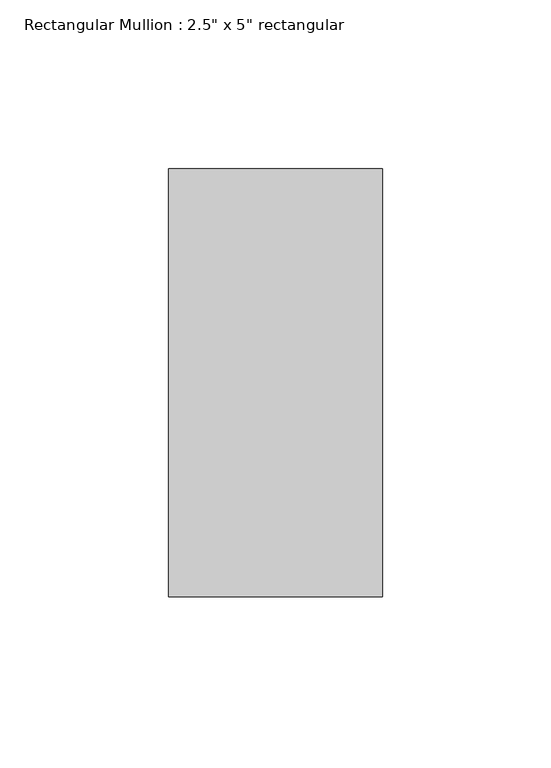
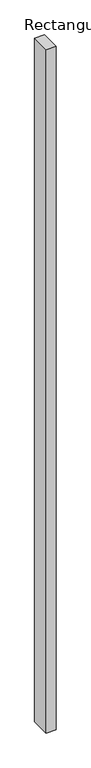
"""IFC4 building model written with IfcOpenShell, lengths in millimetres: member geometry."""

from ifc_helpers import new_model, si_unit, frame, origin, place, context, project, spatial, polyline, outline, extrude, source, transform, mapped, element, save


def member_ab1dc975(model_context):
    return source(origin(), model_context, "Body", "SweptSolid", [
        extrude(outline(polyline([(0.0, 63.5), (0.0, -63.5), (-63.5, -63.5), (-63.5, 63.5), (0.0, 63.5)])), frame((0.0, 0.0, -4640.5080091), z_axis=(0.0, 0.0, 1.0), x_axis=(1.0, 0.0, 0.0)), (0.0, 0.0, 1.0), 4640.5080091),
    ])


if __name__ == "__main__":
    model = new_model("IFC4")
    model_context = context("Model", 3, world=origin())
    ifc_project = project(units=[si_unit("LENGTHUNIT", "METRE", prefix="MILLI")], contexts=[model_context])
    site = spatial("IfcSite", under=ifc_project)
    building = spatial("IfcBuilding", under=site)
    placement = place(None, origin())
    member_shape = member_ab1dc975(model_context)
    element("IfcMember", 1, ObjectType="Rectangular Mullion : 2.5\" x 5\" rectangular", at=placement, inside=building, context=model_context, shape_type="MappedRepresentation", body=[
        mapped(member_shape, transform((0.0, 0.0, 0.0), x_axis=(1.0, 0.0, 0.0), y_axis=(0.0, 1.0, 0.0), z_axis=(0.0, 0.0, 1.0))),
    ])
    save(model, "model.ifc")

# Revit data of these elements
# Type "Rectangular Mullion : 2.5\" x 5\" rectangular"
#   built-in parameter 1007304 = 0.416667 (stored number, unit not read)
#   built-in parameter 1007301 = 0.104167 (stored number, unit not read)
#   built-in parameter 1007300 = 0.104167 (stored number, unit not read)
# Element 1 (IfcMember, "Rectangular Mullion : 2.5\" x 5\" rectangular")
#   Materials on its faces: "Aluminum"
# Materials
#   "Aluminum": class "Metal", colour RGB 247 247 247, transparency 0, Description = "Aluminum 6061", Cost = 0
